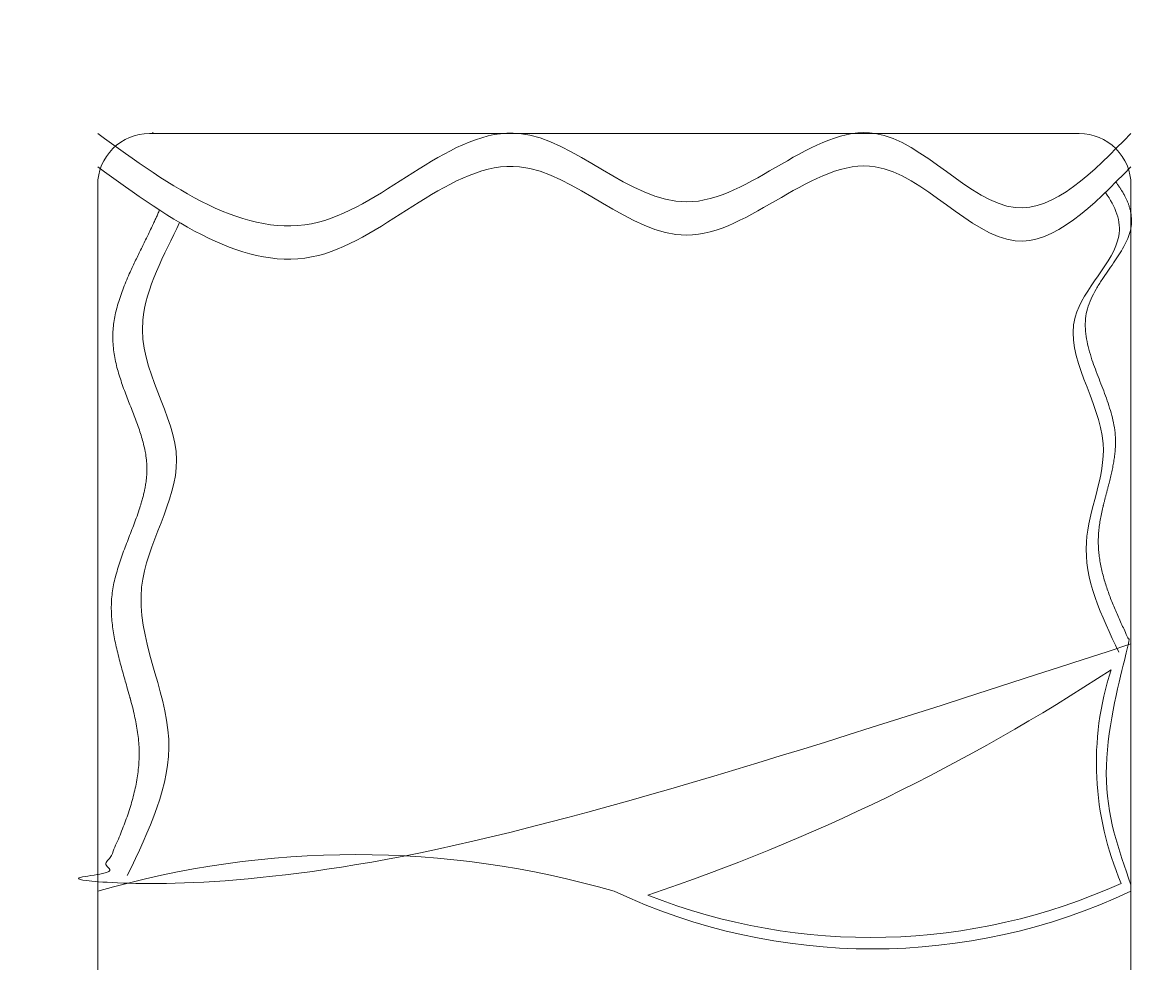
# Model space of a CAD drawing. Units: inches. Extents: x -61 to 1599, y -1316 to 257.
# Tile 188 of 204: x 1088 to 1163, y -391 to -328. Entities that reach past the tile are written whole.
import ezdxf

# ---------------------------------------------------------------- set-up
doc = ezdxf.new("R2010")
doc.units = ezdxf.units.IN
doc.header["$MEASUREMENT"] = 0
doc.layers.add('A-ANNO-DIMS', color=2, linetype='Continuous', lineweight=18)
doc.layers.add('FURNITURE', color=83, linetype='Continuous', lineweight=18)
doc.layers.add('LT', color=8, linetype='Continuous')
doc.styles.get("Standard").update_dxf_attribs({"font": 'arial.ttf'})
doc.dimstyles.get("Standard").update_dxf_attribs({"dimtxt": 0.18, "dimasz": 0.18, "dimexe": 0.18, "dimexo": 0.0625, "dimgap": 0.09, "dimtad": 0, "dimtih": 1, "dimtoh": 1, "dimdec": 0, "dimzin": 0, "dimdsep": 46, "dimlunit": 3, "dimtxsty": 'Standard', "dimcen": 0.09, "dimadec": 0, "dimazin": 0, "dimtfac": 1, "dimtdec": 0, "dimtofl": 0, "dimtmove": 0, "dimatfit": 3, "dimfxl": 1, "dimtolj": 1, "dimtzin": 0, "dimarcsym": 0})

# ---------------------------------------------------------------- blocks, each defined once
blk = doc.blocks.new('*U15')
at = {"layer": 'LT'}
blk.add_line((0, 0.175), (0, -0.175), dxfattribs=at)
for centre, start, end in [((0.509, 0), 160.9983, 199.0017), ((-0.509, 0), 340.9983, 19.0017)]:
    blk.add_arc(centre, 0.539, start, end, dxfattribs=at)
blk = doc.blocks.new('*U16')
at = {"layer": 'LT', "transparency": 16777216}
for p, rotation in [((-66.649, -18.828), 96), ((-66.642, -18.755), 72), ((-66.627, -18.897), 120), ((-66.605, -18.692), 48.00000000000001), ((-66.578, -18.951), 144), ((-66.546, -18.649), 24), ((-66.512, -18.981), 168.0000000000001), ((-66.439, -18.981), 192), ((-66.404, -18.649), 336.0000000000001), ((-66.372, -18.951), 216), ((-66.345, -18.692), 312), ((-66.323, -18.897), 240), ((-66.308, -18.755), 288.0000000000001), ((-66.301, -18.828), 264)]:
    blk.add_blockref('*U15', p, dxfattribs=dict(at, rotation=rotation))
blk.add_blockref('*U15', (-66.475, -18.634), dxfattribs=at)
blk = doc.blocks.new('*U45')
at = {"layer": 'LT'}
blk.add_line((0, 0.175), (0, -0.175), dxfattribs=at)
for centre, start, end in [((0.509, 0), 160.9983, 199.0017), ((-0.509, 0), 340.9983, 19.0017)]:
    blk.add_arc(centre, 0.539, start, end, dxfattribs=at)
blk = doc.blocks.new('*U46')
at = {"layer": 'LT', "transparency": 16777216}
for p, rotation in [((-66.649, -18.828), 96), ((-66.642, -18.755), 72), ((-66.627, -18.897), 120), ((-66.605, -18.692), 48.00000000000001), ((-66.578, -18.951), 144), ((-66.546, -18.649), 24), ((-66.512, -18.981), 168.0000000000001), ((-66.439, -18.981), 192), ((-66.404, -18.649), 336.0000000000001), ((-66.372, -18.951), 216), ((-66.345, -18.692), 312), ((-66.323, -18.897), 240), ((-66.308, -18.755), 288.0000000000001), ((-66.301, -18.828), 264)]:
    blk.add_blockref('*U45', p, dxfattribs=dict(at, rotation=rotation))
blk.add_blockref('*U45', (-66.475, -18.634), dxfattribs=at)
blk = doc.blocks.new('*U9')
at = {"layer": 'LT'}
blk.add_line((0, 0.175), (0, -0.175), dxfattribs=at)
for centre, start, end in [((0.509, 0), 160.9983, 199.0017), ((-0.509, 0), 340.9983, 19.0017)]:
    blk.add_arc(centre, 0.539, start, end, dxfattribs=at)
blk = doc.blocks.new('*U10')
at = {"layer": 'LT', "transparency": 16777216}
for p, rotation in [((-66.649, -18.828), 96), ((-66.642, -18.755), 72), ((-66.627, -18.897), 120), ((-66.605, -18.692), 48.00000000000001), ((-66.578, -18.951), 144), ((-66.546, -18.649), 24), ((-66.512, -18.981), 168.0000000000001), ((-66.439, -18.981), 192), ((-66.404, -18.649), 336.0000000000001), ((-66.372, -18.951), 216), ((-66.345, -18.692), 312), ((-66.323, -18.897), 240), ((-66.308, -18.755), 288.0000000000001), ((-66.301, -18.828), 264)]:
    blk.add_blockref('*U9', p, dxfattribs=dict(at, rotation=rotation))
blk.add_blockref('*U9', (-66.475, -18.634), dxfattribs=at)
blk = doc.blocks.new('*U39')
at = {"layer": 'LT'}
blk.add_line((0, 0.175), (0, -0.175), dxfattribs=at)
for centre, start, end in [((0.509, 0), 160.9983, 199.0017), ((-0.509, 0), 340.9983, 19.0017)]:
    blk.add_arc(centre, 0.539, start, end, dxfattribs=at)
blk = doc.blocks.new('*U40')
at = {"layer": 'LT', "transparency": 16777216}
for p, rotation in [((-66.649, -18.828), 96), ((-66.642, -18.755), 72), ((-66.627, -18.897), 120), ((-66.605, -18.692), 48.00000000000001), ((-66.578, -18.951), 144), ((-66.546, -18.649), 24), ((-66.512, -18.981), 168.0000000000001), ((-66.439, -18.981), 192), ((-66.404, -18.649), 336.0000000000001), ((-66.372, -18.951), 216), ((-66.345, -18.692), 312), ((-66.323, -18.897), 240), ((-66.308, -18.755), 288.0000000000001), ((-66.301, -18.828), 264)]:
    blk.add_blockref('*U39', p, dxfattribs=dict(at, rotation=rotation))
blk.add_blockref('*U39', (-66.475, -18.634), dxfattribs=at)
blk = doc.blocks.new('*U17')
at = {"layer": 'LT'}
blk.add_line((0, 0.412), (0, -0.412), dxfattribs=at)
for centre, start, end in [((1.198, 0), 160.9983, 199.0017), ((-1.198, 0), 340.9983, 19.0017)]:
    blk.add_arc(centre, 1.267, start, end, dxfattribs=at)
blk = doc.blocks.new('*U18')
at = {"layer": 'LT', "transparency": 16777216}
for p, rotation in [((-156.639, -43.959), 48.00000000000001), ((-156.501, -43.858), 24), ((-156.165, -43.858), 336.0000000000001), ((-156.027, -43.959), 312), ((-156.743, -44.278), 96), ((-156.725, -44.108), 72), ((-156.69, -44.441), 120), ((-156.575, -44.569), 144), ((-156.419, -44.639), 168), ((-156.247, -44.639), 192), ((-156.091, -44.569), 216), ((-155.976, -44.441), 240), ((-155.941, -44.108), 288.0000000000001), ((-155.923, -44.278), 264)]:
    blk.add_blockref('*U17', p, dxfattribs=dict(at, rotation=rotation))
blk.add_blockref('*U17', (-156.333, -43.823), dxfattribs=at)
blk = doc.blocks.new('*U33')
at = {"layer": 'LT'}
blk.add_line((0, 0.412), (0, -0.412), dxfattribs=at)
for centre, start, end in [((1.198, 0), 160.9983, 199.0017), ((-1.198, 0), 340.9983, 19.0017)]:
    blk.add_arc(centre, 1.267, start, end, dxfattribs=at)
blk = doc.blocks.new('*U34')
at = {"layer": 'LT', "transparency": 16777216}
for p, rotation in [((-156.639, -43.959), 48.00000000000001), ((-156.501, -43.858), 24), ((-156.165, -43.858), 336.0000000000001), ((-156.027, -43.959), 312), ((-156.743, -44.278), 96), ((-156.725, -44.108), 72), ((-156.69, -44.441), 120), ((-156.575, -44.569), 144), ((-156.419, -44.639), 168), ((-156.247, -44.639), 192), ((-156.091, -44.569), 216), ((-155.976, -44.441), 240), ((-155.941, -44.108), 288.0000000000001), ((-155.923, -44.278), 264)]:
    blk.add_blockref('*U33', p, dxfattribs=dict(at, rotation=rotation))
blk.add_blockref('*U33', (-156.333, -43.823), dxfattribs=at)
blk = doc.blocks.new('*U11')
at = {"layer": 'LT'}
blk.add_line((0, 0.739), (0, -0.739), dxfattribs=at)
for centre, start, end in [((2.147, 0), 160.9983, 199.0017), ((-2.147, 0), 340.9983, 19.0017)]:
    blk.add_arc(centre, 2.27, start, end, dxfattribs=at)
blk = doc.blocks.new('*U12')
at = {"layer": 'LT', "transparency": 16777216}
for p, rotation in [((-280.791, -78.801), 48.00000000000001), ((-280.542, -78.621), 23.99999999999999), ((-279.941, -78.621), 336.0000000000001), ((-279.692, -78.801), 312), ((-280.977, -79.373), 96), ((-280.945, -79.067), 72), ((-280.882, -79.665), 120), ((-280.676, -79.894), 144), ((-280.395, -80.019), 168), ((-280.088, -80.019), 191.9999999999999), ((-279.807, -79.894), 216), ((-279.602, -79.665), 240), ((-279.539, -79.067), 288.0000000000001), ((-279.507, -79.373), 264)]:
    blk.add_blockref('*U11', p, dxfattribs=dict(at, rotation=rotation))
blk.add_blockref('*U11', (-280.242, -78.557), dxfattribs=at)
blk = doc.blocks.new('*U28')
at = {"layer": 'LT'}
blk.add_line((0, 0.412), (0, -0.412), dxfattribs=at)
for centre, start, end in [((1.198, 0), 160.9983, 199.0017), ((-1.198, 0), 340.9983, 19.0017)]:
    blk.add_arc(centre, 1.267, start, end, dxfattribs=at)
blk = doc.blocks.new('*U44')
at = {"layer": 'LT', "transparency": 16777216}
for p, rotation in [((-156.639, -43.959), 48.00000000000001), ((-156.501, -43.858), 24), ((-156.165, -43.858), 336.0000000000001), ((-156.027, -43.959), 312), ((-156.743, -44.278), 96), ((-156.725, -44.108), 72), ((-156.69, -44.441), 120), ((-156.575, -44.569), 144), ((-156.419, -44.639), 168), ((-156.247, -44.639), 192), ((-156.091, -44.569), 216), ((-155.976, -44.441), 240), ((-155.941, -44.108), 288.0000000000001), ((-155.923, -44.278), 264)]:
    blk.add_blockref('*U28', p, dxfattribs=dict(at, rotation=rotation))
blk.add_blockref('*U28', (-156.333, -43.823), dxfattribs=at)
blk = doc.blocks.new('*U13')
at = {"layer": 'LT'}
blk.add_line((0, 0.412), (0, -0.412), dxfattribs=at)
for centre, start, end in [((1.198, 0), 160.9983, 199.0017), ((-1.198, 0), 340.9983, 19.0017)]:
    blk.add_arc(centre, 1.267, start, end, dxfattribs=at)
blk = doc.blocks.new('*U14')
at = {"layer": 'LT', "transparency": 16777216}
for p, rotation in [((-156.639, -43.959), 48.00000000000001), ((-156.501, -43.858), 24), ((-156.165, -43.858), 336.0000000000001), ((-156.027, -43.959), 312), ((-156.743, -44.278), 96), ((-156.725, -44.108), 72), ((-156.69, -44.441), 120), ((-156.575, -44.569), 144), ((-156.419, -44.639), 168), ((-156.247, -44.639), 192), ((-156.091, -44.569), 216), ((-155.976, -44.441), 240), ((-155.941, -44.108), 288.0000000000001), ((-155.923, -44.278), 264)]:
    blk.add_blockref('*U13', p, dxfattribs=dict(at, rotation=rotation))
blk.add_blockref('*U13', (-156.333, -43.823), dxfattribs=at)
blk = doc.blocks.new('*U19')
at = {"layer": 'LT'}
blk.add_line((0, 0.175), (0, -0.175), dxfattribs=at)
for centre, start, end in [((0.509, 0), 160.9983, 199.0017), ((-0.509, 0), 340.9983, 19.0017)]:
    blk.add_arc(centre, 0.539, start, end, dxfattribs=at)
blk = doc.blocks.new('*U6')
at = {"layer": 'LT', "transparency": 16777216}
for p, rotation in [((-66.649, -18.828), 96), ((-66.642, -18.755), 72), ((-66.627, -18.897), 120), ((-66.605, -18.692), 48.00000000000001), ((-66.578, -18.951), 144), ((-66.546, -18.649), 24), ((-66.512, -18.981), 168.0000000000001), ((-66.439, -18.981), 192), ((-66.404, -18.649), 336.0000000000001), ((-66.372, -18.951), 216), ((-66.345, -18.692), 312), ((-66.323, -18.897), 240), ((-66.308, -18.755), 288.0000000000001), ((-66.301, -18.828), 264)]:
    blk.add_blockref('*U19', p, dxfattribs=dict(at, rotation=rotation))
blk.add_blockref('*U19', (-66.475, -18.634), dxfattribs=at)
blk = doc.blocks.new('*U35')
at = {"layer": 'LT'}
blk.add_line((0, 0.175), (0, -0.175), dxfattribs=at)
for centre, start, end in [((0.509, 0), 160.9983, 199.0017), ((-0.509, 0), 340.9983, 19.0017)]:
    blk.add_arc(centre, 0.539, start, end, dxfattribs=at)
blk = doc.blocks.new('*U36')
at = {"layer": 'LT', "transparency": 16777216}
for p, rotation in [((-66.649, -18.828), 96), ((-66.642, -18.755), 72), ((-66.627, -18.897), 120), ((-66.605, -18.692), 48.00000000000001), ((-66.578, -18.951), 144), ((-66.546, -18.649), 24), ((-66.512, -18.981), 168.0000000000001), ((-66.439, -18.981), 192), ((-66.404, -18.649), 336.0000000000001), ((-66.372, -18.951), 216), ((-66.345, -18.692), 312), ((-66.323, -18.897), 240), ((-66.308, -18.755), 288.0000000000001), ((-66.301, -18.828), 264)]:
    blk.add_blockref('*U35', p, dxfattribs=dict(at, rotation=rotation))
blk.add_blockref('*U35', (-66.475, -18.634), dxfattribs=at)
blk = doc.blocks.new('*U7')
at = {"layer": 'LT'}
blk.add_line((0, 0.175), (0, -0.175), dxfattribs=at)
for centre, start, end in [((0.509, 0), 160.9983, 199.0017), ((-0.509, 0), 340.9983, 19.0017)]:
    blk.add_arc(centre, 0.539, start, end, dxfattribs=at)
blk = doc.blocks.new('*U8')
at = {"layer": 'LT', "transparency": 16777216}
for p, rotation in [((-66.649, -18.828), 96), ((-66.642, -18.755), 72), ((-66.627, -18.897), 120), ((-66.605, -18.692), 48.00000000000001), ((-66.578, -18.951), 144), ((-66.546, -18.649), 24), ((-66.512, -18.981), 168.0000000000001), ((-66.439, -18.981), 192), ((-66.404, -18.649), 336.0000000000001), ((-66.372, -18.951), 216), ((-66.345, -18.692), 312), ((-66.323, -18.897), 240), ((-66.308, -18.755), 288.0000000000001), ((-66.301, -18.828), 264)]:
    blk.add_blockref('*U7', p, dxfattribs=dict(at, rotation=rotation))
blk.add_blockref('*U7', (-66.475, -18.634), dxfattribs=at)
blk = doc.blocks.new('*U37')
at = {"layer": 'LT'}
blk.add_line((0, 0.175), (0, -0.175), dxfattribs=at)
for centre, start, end in [((0.509, 0), 160.9983, 199.0017), ((-0.509, 0), 340.9983, 19.0017)]:
    blk.add_arc(centre, 0.539, start, end, dxfattribs=at)
blk = doc.blocks.new('*U38')
at = {"layer": 'LT', "transparency": 16777216}
for p, rotation in [((-66.649, -18.828), 96), ((-66.642, -18.755), 72), ((-66.627, -18.897), 120), ((-66.605, -18.692), 48.00000000000001), ((-66.578, -18.951), 144), ((-66.546, -18.649), 24), ((-66.512, -18.981), 168.0000000000001), ((-66.439, -18.981), 192), ((-66.404, -18.649), 336.0000000000001), ((-66.372, -18.951), 216), ((-66.345, -18.692), 312), ((-66.323, -18.897), 240), ((-66.308, -18.755), 288.0000000000001), ((-66.301, -18.828), 264)]:
    blk.add_blockref('*U37', p, dxfattribs=dict(at, rotation=rotation))
blk.add_blockref('*U37', (-66.475, -18.634), dxfattribs=at)
blk = doc.blocks.new('*U3')
at = {"layer": 'LT'}
blk.add_line((0, 0.175), (0, -0.175), dxfattribs=at)
for centre, start, end in [((0.509, 0), 160.9983, 199.0017), ((-0.509, 0), 340.9983, 19.0017)]:
    blk.add_arc(centre, 0.539, start, end, dxfattribs=at)
blk = doc.blocks.new('*U4')
at = {"layer": 'LT', "transparency": 16777216}
for p, rotation in [((-66.649, -18.828), 96), ((-66.642, -18.755), 72), ((-66.627, -18.897), 120), ((-66.605, -18.692), 48.00000000000001), ((-66.578, -18.951), 144), ((-66.546, -18.649), 24), ((-66.512, -18.981), 168.0000000000001), ((-66.439, -18.981), 192), ((-66.404, -18.649), 336.0000000000001), ((-66.372, -18.951), 216), ((-66.345, -18.692), 312), ((-66.323, -18.897), 240), ((-66.308, -18.755), 288.0000000000001), ((-66.301, -18.828), 264)]:
    blk.add_blockref('*U3', p, dxfattribs=dict(at, rotation=rotation))
blk.add_blockref('*U3', (-66.475, -18.634), dxfattribs=at)
blk = doc.blocks.new('*U20')
at = {"layer": 'LT'}
blk.add_line((0, 0.175), (0, -0.175), dxfattribs=at)
for centre, start, end in [((0.509, 0), 160.9983, 199.0017), ((-0.509, 0), 340.9983, 19.0017)]:
    blk.add_arc(centre, 0.539, start, end, dxfattribs=at)
blk = doc.blocks.new('*U21')
at = {"layer": 'LT', "transparency": 16777216}
for p, rotation in [((-66.649, -18.828), 96), ((-66.642, -18.755), 72), ((-66.627, -18.897), 120), ((-66.605, -18.692), 48.00000000000001), ((-66.578, -18.951), 144), ((-66.546, -18.649), 24), ((-66.512, -18.981), 168.0000000000001), ((-66.439, -18.981), 192), ((-66.404, -18.649), 336.0000000000001), ((-66.372, -18.951), 216), ((-66.345, -18.692), 312), ((-66.323, -18.897), 240), ((-66.308, -18.755), 288.0000000000001), ((-66.301, -18.828), 264)]:
    blk.add_blockref('*U20', p, dxfattribs=dict(at, rotation=rotation))
blk.add_blockref('*U20', (-66.475, -18.634), dxfattribs=at)
blk = doc.blocks.new('*U52')
at = {"layer": 'LT'}
blk.add_line((0, 0.175), (0, -0.175), dxfattribs=at)
for centre, start, end in [((0.509, 0), 160.9983, 199.0017), ((-0.509, 0), 340.9983, 19.0017)]:
    blk.add_arc(centre, 0.539, start, end, dxfattribs=at)
blk = doc.blocks.new('*U53')
at = {"layer": 'LT', "transparency": 16777216}
for p, rotation in [((-66.649, -18.828), 96), ((-66.642, -18.755), 72), ((-66.627, -18.897), 120), ((-66.605, -18.692), 48.00000000000001), ((-66.578, -18.951), 144), ((-66.546, -18.649), 24), ((-66.512, -18.981), 168.0000000000001), ((-66.439, -18.981), 192), ((-66.404, -18.649), 336.0000000000001), ((-66.372, -18.951), 216), ((-66.345, -18.692), 312), ((-66.323, -18.897), 240), ((-66.308, -18.755), 288.0000000000001), ((-66.301, -18.828), 264)]:
    blk.add_blockref('*U52', p, dxfattribs=dict(at, rotation=rotation))
blk.add_blockref('*U52', (-66.475, -18.634), dxfattribs=at)
blk = doc.blocks.new('*U29')
at = {"layer": 'LT'}
blk.add_line((0, 0.175), (0, -0.175), dxfattribs=at)
for centre, start, end in [((0.509, 0), 160.9983, 199.0017), ((-0.509, 0), 340.9983, 19.0017)]:
    blk.add_arc(centre, 0.539, start, end, dxfattribs=at)
blk = doc.blocks.new('*U30')
at = {"layer": 'LT', "transparency": 16777216}
for p, rotation in [((-66.649, -18.828), 96), ((-66.642, -18.755), 72), ((-66.627, -18.897), 120), ((-66.605, -18.692), 48.00000000000001), ((-66.578, -18.951), 144), ((-66.546, -18.649), 24), ((-66.512, -18.981), 168.0000000000001), ((-66.439, -18.981), 192), ((-66.404, -18.649), 336.0000000000001), ((-66.372, -18.951), 216), ((-66.345, -18.692), 312), ((-66.323, -18.897), 240), ((-66.308, -18.755), 288.0000000000001), ((-66.301, -18.828), 264)]:
    blk.add_blockref('*U29', p, dxfattribs=dict(at, rotation=rotation))
blk.add_blockref('*U29', (-66.475, -18.634), dxfattribs=at)
blk = doc.blocks.new('*U5')
at = {"layer": 'LT'}
blk.add_line((0, 0.412), (0, -0.412), dxfattribs=at)
for centre, start, end in [((1.198, 0), 160.9983, 199.0017), ((-1.198, 0), 340.9983, 19.0017)]:
    blk.add_arc(centre, 1.267, start, end, dxfattribs=at)
blk = doc.blocks.new('*U47')
at = {"layer": 'LT', "transparency": 16777216}
for p, rotation in [((-156.639, -43.959), 48.00000000000001), ((-156.501, -43.858), 24), ((-156.165, -43.858), 336.0000000000001), ((-156.027, -43.959), 312), ((-156.743, -44.278), 96), ((-156.725, -44.108), 72), ((-156.69, -44.441), 120), ((-156.575, -44.569), 144), ((-156.419, -44.639), 168), ((-156.247, -44.639), 192), ((-156.091, -44.569), 216), ((-155.976, -44.441), 240), ((-155.941, -44.108), 288.0000000000001), ((-155.923, -44.278), 264)]:
    blk.add_blockref('*U5', p, dxfattribs=dict(at, rotation=rotation))
blk.add_blockref('*U5', (-156.333, -43.823), dxfattribs=at)
blk = doc.blocks.new('*U22')
at = {"layer": 'LT'}
blk.add_line((0, 0.412), (0, -0.412), dxfattribs=at)
for centre, start, end in [((1.198, 0), 160.9983, 199.0017), ((-1.198, 0), 340.9983, 19.0017)]:
    blk.add_arc(centre, 1.267, start, end, dxfattribs=at)
blk = doc.blocks.new('*U23')
at = {"layer": 'LT', "transparency": 16777216}
for p, rotation in [((-156.639, -43.959), 48.00000000000001), ((-156.501, -43.858), 24), ((-156.165, -43.858), 336.0000000000001), ((-156.027, -43.959), 312), ((-156.743, -44.278), 96), ((-156.725, -44.108), 72), ((-156.69, -44.441), 120), ((-156.575, -44.569), 144), ((-156.419, -44.639), 168), ((-156.247, -44.639), 192), ((-156.091, -44.569), 216), ((-155.976, -44.441), 240), ((-155.941, -44.108), 288.0000000000001), ((-155.923, -44.278), 264)]:
    blk.add_blockref('*U22', p, dxfattribs=dict(at, rotation=rotation))
blk.add_blockref('*U22', (-156.333, -43.823), dxfattribs=at)
blk = doc.blocks.new('*U54')
at = {"layer": 'LT'}
blk.add_line((0, 0.739), (0, -0.739), dxfattribs=at)
for centre, start, end in [((2.147, 0), 160.9983, 199.0017), ((-2.147, 0), 340.9983, 19.0017)]:
    blk.add_arc(centre, 2.27, start, end, dxfattribs=at)
blk = doc.blocks.new('*U41')
at = {"layer": 'LT', "transparency": 16777216}
for p, rotation in [((-280.791, -78.801), 48.00000000000001), ((-280.542, -78.621), 23.99999999999999), ((-279.941, -78.621), 336.0000000000001), ((-279.692, -78.801), 312), ((-280.977, -79.373), 96), ((-280.945, -79.067), 72), ((-280.882, -79.665), 120), ((-280.676, -79.894), 144), ((-280.395, -80.019), 168), ((-280.088, -80.019), 191.9999999999999), ((-279.807, -79.894), 216), ((-279.602, -79.665), 240), ((-279.539, -79.067), 288.0000000000001), ((-279.507, -79.373), 264)]:
    blk.add_blockref('*U54', p, dxfattribs=dict(at, rotation=rotation))
blk.add_blockref('*U54', (-280.242, -78.557), dxfattribs=at)
blk = doc.blocks.new('*U42')
at = {"layer": 'LT'}
blk.add_line((0, 0.412), (0, -0.412), dxfattribs=at)
for centre, start, end in [((1.198, 0), 160.9983, 199.0017), ((-1.198, 0), 340.9983, 19.0017)]:
    blk.add_arc(centre, 1.267, start, end, dxfattribs=at)
blk = doc.blocks.new('*U43')
at = {"layer": 'LT', "transparency": 16777216}
for p, rotation in [((-156.639, -43.959), 48.00000000000001), ((-156.501, -43.858), 24), ((-156.165, -43.858), 336.0000000000001), ((-156.027, -43.959), 312), ((-156.743, -44.278), 96), ((-156.725, -44.108), 72), ((-156.69, -44.441), 120), ((-156.575, -44.569), 144), ((-156.419, -44.639), 168), ((-156.247, -44.639), 192), ((-156.091, -44.569), 216), ((-155.976, -44.441), 240), ((-155.941, -44.108), 288.0000000000001), ((-155.923, -44.278), 264)]:
    blk.add_blockref('*U42', p, dxfattribs=dict(at, rotation=rotation))
blk.add_blockref('*U42', (-156.333, -43.823), dxfattribs=at)
blk = doc.blocks.new('*U31')
at = {"layer": 'LT'}
blk.add_line((0, 0.412), (0, -0.412), dxfattribs=at)
for centre, start, end in [((1.198, 0), 160.9983, 199.0017), ((-1.198, 0), 340.9983, 19.0017)]:
    blk.add_arc(centre, 1.267, start, end, dxfattribs=at)
blk = doc.blocks.new('*U32')
at = {"layer": 'LT', "transparency": 16777216}
for p, rotation in [((-156.639, -43.959), 48.00000000000001), ((-156.501, -43.858), 24), ((-156.165, -43.858), 336.0000000000001), ((-156.027, -43.959), 312), ((-156.743, -44.278), 96), ((-156.725, -44.108), 72), ((-156.69, -44.441), 120), ((-156.575, -44.569), 144), ((-156.419, -44.639), 168), ((-156.247, -44.639), 192), ((-156.091, -44.569), 216), ((-155.976, -44.441), 240), ((-155.941, -44.108), 288.0000000000001), ((-155.923, -44.278), 264)]:
    blk.add_blockref('*U31', p, dxfattribs=dict(at, rotation=rotation))
blk.add_blockref('*U31', (-156.333, -43.823), dxfattribs=at)
blk = doc.blocks.new('*U48')
at = {"layer": 'LT'}
blk.add_line((0, 0.175), (0, -0.175), dxfattribs=at)
for centre, start, end in [((0.509, 0), 160.9983, 199.0017), ((-0.509, 0), 340.9983, 19.0017)]:
    blk.add_arc(centre, 0.539, start, end, dxfattribs=at)
blk = doc.blocks.new('*U49')
at = {"layer": 'LT', "transparency": 16777216}
for p, rotation in [((-66.649, -18.828), 96), ((-66.642, -18.755), 72), ((-66.627, -18.897), 120), ((-66.605, -18.692), 48.00000000000001), ((-66.578, -18.951), 144), ((-66.546, -18.649), 24), ((-66.512, -18.981), 168.0000000000001), ((-66.439, -18.981), 192), ((-66.404, -18.649), 336.0000000000001), ((-66.372, -18.951), 216), ((-66.345, -18.692), 312), ((-66.323, -18.897), 240), ((-66.308, -18.755), 288.0000000000001), ((-66.301, -18.828), 264)]:
    blk.add_blockref('*U48', p, dxfattribs=dict(at, rotation=rotation))
blk.add_blockref('*U48', (-66.475, -18.634), dxfattribs=at)
blk = doc.blocks.new('*U24')
at = {"layer": 'LT'}
blk.add_line((0, 0.175), (0, -0.175), dxfattribs=at)
for centre, start, end in [((0.509, 0), 160.9983, 199.0017), ((-0.509, 0), 340.9983, 19.0017)]:
    blk.add_arc(centre, 0.539, start, end, dxfattribs=at)
blk = doc.blocks.new('*U25')
at = {"layer": 'LT', "transparency": 16777216}
for p, rotation in [((-66.649, -18.828), 96), ((-66.642, -18.755), 72), ((-66.627, -18.897), 120), ((-66.605, -18.692), 48.00000000000001), ((-66.578, -18.951), 144), ((-66.546, -18.649), 24), ((-66.512, -18.981), 168.0000000000001), ((-66.439, -18.981), 192), ((-66.404, -18.649), 336.0000000000001), ((-66.372, -18.951), 216), ((-66.345, -18.692), 312), ((-66.323, -18.897), 240), ((-66.308, -18.755), 288.0000000000001), ((-66.301, -18.828), 264)]:
    blk.add_blockref('*U24', p, dxfattribs=dict(at, rotation=rotation))
blk.add_blockref('*U24', (-66.475, -18.634), dxfattribs=at)
blk = doc.blocks.new('*U50')
at = {"layer": 'LT'}
blk.add_line((0, 0.175), (0, -0.175), dxfattribs=at)
for centre, start, end in [((0.509, 0), 160.9983, 199.0017), ((-0.509, 0), 340.9983, 19.0017)]:
    blk.add_arc(centre, 0.539, start, end, dxfattribs=at)
blk = doc.blocks.new('*U51')
at = {"layer": 'LT', "transparency": 16777216}
for p, rotation in [((-66.649, -18.828), 96), ((-66.642, -18.755), 72), ((-66.627, -18.897), 120), ((-66.605, -18.692), 48.00000000000001), ((-66.578, -18.951), 144), ((-66.546, -18.649), 24), ((-66.512, -18.981), 168.0000000000001), ((-66.439, -18.981), 192), ((-66.404, -18.649), 336.0000000000001), ((-66.372, -18.951), 216), ((-66.345, -18.692), 312), ((-66.323, -18.897), 240), ((-66.308, -18.755), 288.0000000000001), ((-66.301, -18.828), 264)]:
    blk.add_blockref('*U50', p, dxfattribs=dict(at, rotation=rotation))
blk.add_blockref('*U50', (-66.475, -18.634), dxfattribs=at)
blk = doc.blocks.new('*U26')
at = {"layer": 'LT'}
blk.add_line((0, 0.175), (0, -0.175), dxfattribs=at)
for centre, start, end in [((0.509, 0), 160.9983, 199.0017), ((-0.509, 0), 340.9983, 19.0017)]:
    blk.add_arc(centre, 0.539, start, end, dxfattribs=at)
blk = doc.blocks.new('*U27')
at = {"layer": 'LT', "transparency": 16777216}
for p, rotation in [((-66.649, -18.828), 96), ((-66.642, -18.755), 72), ((-66.627, -18.897), 120), ((-66.605, -18.692), 48.00000000000001), ((-66.578, -18.951), 144), ((-66.546, -18.649), 24), ((-66.512, -18.981), 168.0000000000001), ((-66.439, -18.981), 192), ((-66.404, -18.649), 336.0000000000001), ((-66.372, -18.951), 216), ((-66.345, -18.692), 312), ((-66.323, -18.897), 240), ((-66.308, -18.755), 288.0000000000001), ((-66.301, -18.828), 264)]:
    blk.add_blockref('*U26', p, dxfattribs=dict(at, rotation=rotation))
blk.add_blockref('*U26', (-66.475, -18.634), dxfattribs=at)
blk = doc.blocks.new('BED-DOUBLE')
for p, q in [((1.272, 20.467), (70.263, 20.467)), ((1.272, 19.317), (70.263, 19.317)), ((10.471, 1.379), (10.471, 16.557)), ((34.388, 16.557), (10.471, 16.557)), ((10.471, 16.557), (13.35, 15.18)), ((10.471, 16.557), (14.039, 13.107)), ((10.471, 16.557), (12.454, 13.305)), ((34.388, 16.557), (30.82, 13.107)), ((34.388, 16.557), (31.508, 15.18)), ((34.388, 16.557), (32.405, 13.305)), ((37.147, 1.379), (37.147, 16.557)), ((61.064, 16.557), (37.147, 16.557)), ((37.147, 16.557), (40.027, 15.18)), ((37.147, 16.557), (40.715, 13.107)), ((37.147, 16.557), (39.13, 13.305)), ((61.064, 16.557), (57.496, 13.107)), ((61.064, 16.557), (58.185, 15.18)), ((61.064, 16.557), (59.081, 13.305)), ((13.35, 15.18), (13.35, 14.829)), ((31.508, 15.18), (31.508, 14.829)), ((40.027, 15.18), (40.027, 14.829)), ((58.185, 15.18), (58.185, 14.829)), ((12.454, 13.305), (12.454, 12.955)), ((14.052, 13.149), (14.052, 12.324)), ((30.806, 13.149), (30.806, 12.324)), ((32.405, 13.305), (32.405, 12.955)), ((39.13, 13.305), (39.13, 12.955)), ((40.729, 13.149), (40.729, 12.324)), ((57.483, 13.149), (57.483, 12.324)), ((59.081, 13.305), (59.081, 12.955)), ((22.429, 8.968), (22.429, 10.447)), ((49.106, 8.968), (49.106, 10.447)), ((14.052, 4.788), (14.052, 5.613)), ((30.806, 4.788), (30.806, 5.613)), ((40.729, 4.788), (40.729, 5.613)), ((57.483, 4.788), (57.483, 5.613)), ((10.471, 1.379), (14.039, 4.83)), ((10.471, 1.379), (12.454, 4.631)), ((12.454, 4.631), (12.454, 4.982)), ((34.388, 1.379), (30.82, 4.83)), ((32.405, 4.631), (32.405, 4.982)), ((34.388, 1.379), (32.405, 4.631)), ((37.147, 1.379), (40.715, 4.83)), ((37.147, 1.379), (39.13, 4.631)), ((39.13, 4.631), (39.13, 4.982)), ((61.064, 1.379), (57.496, 4.83)), ((59.081, 4.631), (59.081, 4.982)), ((61.064, 1.379), (59.081, 4.631)), ((13.35, 2.756), (13.35, 3.107)), ((31.508, 2.756), (31.508, 3.107)), ((40.027, 2.756), (40.027, 3.107)), ((58.185, 2.756), (58.185, 3.107)), ((10.471, 1.379), (13.35, 2.756)), ((34.388, 1.379), (31.508, 2.756)), ((37.147, 1.379), (40.027, 2.756)), ((61.064, 1.379), (58.185, 2.756)), ((34.388, 1.379), (34.388, 1.379)), ((61.064, 1.379), (61.064, 1.379))]:
    blk.add_line(p, q)
for points in [[(1.272, 88.537), (1.272, 3.449, 0.414214), (4.722, 0), (66.813, 0, 0.414214), (70.263, 3.449), (70.263, 88.537, 0.414214), (66.813, 91.987), (4.722, 91.987, 0.414214)], [(38.01, 41.126, 0.064396), (68.933, 56.181, 0.181766), (69.614, 41.916, -0.202767)], [(13.35, 15.18, 0.167358), (13.35, 14.829, 0.167358)], [(40.027, 15.18, 0.167358), (40.027, 14.829, 0.167358)], [(12.454, 13.305, 0.167358), (12.454, 12.955, 0.167358)], [(14.052, 13.149, 0.167358), (14.052, 12.324, 0.167358)], [(30.806, 12.324, 0.167358), (30.806, 13.149, 0.167358)], [(32.405, 12.955, 0.167358), (32.405, 13.305, 0.167358)], [(39.13, 13.305, 0.167358), (39.13, 12.955, 0.167358)], [(40.729, 13.149, 0.167358), (40.729, 12.324, 0.167358)], [(57.483, 12.324, 0.167358), (57.483, 13.149, 0.167358)], [(59.081, 12.955, 0.167358), (59.081, 13.305, 0.167358)], [(22.429, 8.968, 0.167358), (22.429, 10.447, 0.167358)], [(49.106, 8.968, 0.167358), (49.106, 10.447, 0.167358)], [(14.052, 5.613, 0.167358), (14.052, 4.788, 0.167358)], [(30.806, 4.788, 0.167358), (30.806, 5.613, 0.167358)], [(40.729, 5.613, 0.167358), (40.729, 4.788, 0.167358)], [(57.483, 4.788, 0.167358), (57.483, 5.613, 0.167358)], [(12.454, 4.982, 0.167358), (12.454, 4.631, 0.167358)], [(32.405, 4.631, 0.167358), (32.405, 4.982, 0.167358)], [(39.13, 4.982, 0.167358), (39.13, 4.631, 0.167358)], [(59.081, 4.631, 0.167358), (59.081, 4.982, 0.167358)], [(13.35, 3.107, 0.167358), (13.35, 2.756, 0.167358)], [(31.508, 2.756, 0.167358), (31.508, 3.107, 0.167358)], [(40.027, 3.107, 0.167358), (40.027, 2.756, 0.167358)], [(58.185, 2.756, 0.167358), (58.185, 3.107, 0.167358)]]:
    blk.add_lwpolyline(points, format="xyb", close=True)
blk.add_lwpolyline([(70.263, 41.387, -0.22309), (35.767, 41.387, 0.142156), (1.272, 41.387)], format="xyb")
for points in [[(34.388, 16.557), (34.388, 1.379), (10.471, 1.379), (10.471, 16.557), (34.388, 16.557), (34.388, 1.379), (10.471, 1.379)], [(61.064, 16.557), (61.064, 1.379), (37.147, 1.379)]]:
    blk.add_lwpolyline(points)
for centre, radius in [((13.35, 15.18), 0.351), ((31.508, 15.18), 0.351), ((40.027, 15.18), 0.351), ((58.185, 15.18), 0.351), ((12.454, 13.305), 0.351), ((14.052, 13.149), 0.825), ((30.806, 13.149), 0.825), ((32.405, 13.305), 0.351), ((39.13, 13.305), 0.351), ((40.729, 13.149), 0.825), ((57.483, 13.149), 0.825), ((59.081, 13.305), 0.351), ((22.429, 8.968), 1.982), ((49.106, 8.968), 1.982), ((22.429, 8.968), 1.478), ((49.106, 8.968), 1.478), ((14.052, 4.788), 0.825), ((30.806, 4.788), 0.825), ((40.729, 4.788), 0.825), ((57.483, 4.788), 0.825), ((12.454, 4.631), 0.351), ((32.405, 4.631), 0.351), ((39.13, 4.631), 0.351), ((59.081, 4.631), 0.351), ((13.35, 2.756), 0.351), ((31.508, 2.756), 0.351), ((40.027, 2.756), 0.351), ((58.185, 2.756), 0.351)]:
    blk.add_circle(centre, radius)
for centre, radius, start, end in [((-16.003, 8.968), 27.54, 344.0046, 15.9954), ((22.429, 74.54), 59.203, 258.34678, 281.65322), ((60.861, 8.968), 27.54, 164.0046, 195.9954), ((10.674, 8.968), 27.54, 344.0046, 15.9954), ((49.106, 74.54), 59.203, 258.34678, 281.65322), ((87.538, 8.968), 27.54, 164.0046, 195.9954), ((32.017, 15.005), 0.539, 160.9983, 199.0017), ((30.999, 15.005), 0.539, 340.9983, 19.0017), ((58.694, 15.005), 0.539, 160.9983, 199.0017), ((57.675, 15.005), 0.539, 340.9983, 19.0017), ((22.429, -56.603), 59.203, 78.34678, 101.65322), ((49.106, -56.603), 59.203, 78.34678, 101.65322)]:
    blk.add_arc(centre, radius, start, end)
for points, knots in [([(70.263, 91.987), (67.707, 89.379), (62.206, 83.764), (52.487, 96.724), (40.92, 82.741), (28.609, 96.737), (15.695, 81.527), (6.205, 88.409), (1.272, 91.987)], [0, 0, 0, 0, 9.176033, 19.753992, 33.150145, 45.209422, 59.881559, 75.764594, 75.764594, 75.764594, 75.764594]), ([(70.263, 89.765), (67.707, 87.157), (62.206, 81.542), (52.487, 94.502), (40.92, 80.519), (28.609, 94.515), (15.695, 79.305), (6.205, 86.187), (1.272, 89.765)], [0, 0, 0, 0, 9.176033, 19.753992, 33.150145, 45.209422, 59.881559, 75.764594, 75.764594, 75.764594, 75.764594]), ([(69.451, 57.362), (68.289, 59.79), (66.113, 64.336), (70.043, 71.905), (64.118, 79.112), (70.314, 84.4), (69.244, 87.088), (68.552, 88.052)], [0, 0, 0, 0, 6.649676, 12.451782, 19.973966, 25.324174, 28.349676, 28.349676, 28.349676, 28.349676]), ([(3.252, 42.437), (4.702, 45.448), (7.724, 51.72), (2.116, 61.25), (8.808, 70.52), (2.434, 77.934), (5.722, 83.908), (6.746, 86.037)], [0, 0, 0, 0, 8.27671, 17.241866, 24.903358, 33.244933, 38.427294, 38.427294, 38.427294, 38.427294])]:
    blk.add_open_spline(points, degree=3, knots=knots)
blk.add_open_spline([(5.011, 91.987), (4.986, 92.006), (4.961, 92.025), (4.936, 92.044)], degree=3)
for points, weights, knots in [([(70.263, 41.825), (68.018, 47.029), (68.018, 52.696), (70.263, 57.9), (69.1, 60.328), (66.924, 64.874), (70.854, 72.444), (64.929, 79.65), (71.186, 84.991), (70.014, 87.727), (69.253, 88.741)], [1, 0.945466318698, 0.945466318698, 1, 1, 1, 1, 1, 1, 1, 1], [0, 0, 0, 0, 0.814571, 0.814571, 0.814571, 7.464247, 13.266353, 20.788537, 26.138745, 29.321895, 29.321895, 29.321895, 29.321895]), ([(70.263, 57.9), (59.862, 50.943), (48.595, 45.5), (36.681, 41.677), (36.463, 41.771), (36.247, 41.868), (36.032, 41.966), (24.597, 45.284), (12.692, 45.258), (1.272, 41.889), (2.723, 44.9), (5.745, 51.172), (0.137, 60.702), (6.828, 69.972), (0.109, 77.787), (4.354, 84.383), (5.398, 86.876)], [1, 0.993520320424, 0.993520320424, 1, 0.99997444972, 0.99997444972, 1, 0.973174868659, 0.973174868659, 1, 1, 1, 1, 1, 1, 1, 1], [0, 0, 0, 0, 0.279074, 0.279074, 0.279074, 0.296584, 0.296584, 0.296584, 0.865868, 0.865868, 0.865868, 9.142578, 18.107734, 25.769226, 34.110801, 40.441511, 40.441511, 40.441511, 40.441511])]:
    blk.add_rational_spline(points, weights, degree=3, knots=knots)
for name, p in [('*U40', (79.825, 33.99)), ('*U30', (106.502, 33.99)), ('*U46', (78.929, 32.115)), ('*U34', (170.385, 57.384)), ('*U21', (105.605, 32.115)), ('*U23', (197.062, 57.384))]:
    blk.add_blockref(name, p)
at = {"extrusion": (0, 0, -1), "zscale": -1}
for name, p in [('*U36', (34.967, 33.99)), ('*U25', (8.291, 33.99)), ('*U14', (125.527, 57.384)), ('*U38', (34.07, 32.115)), ('*U32', (98.85, 57.384)), ('*U27', (7.394, 32.115))]:
    blk.add_blockref(name, p, dxfattribs=at)
at = {"rotation": 180}
for name, p in [('*U12', (-257.812, -70.328)), ('*U41', (-231.136, -70.328)), ('*U44', (-125.527, -39.447)), ('*U43', (-98.85, -39.447)), ('*U8', (-34.07, -14.178)), ('*U51', (-7.394, -14.178)), ('*U6', (-34.967, -16.053)), ('*U49', (-8.291, -16.053))]:
    blk.add_blockref(name, p, dxfattribs=at)
at = {"extrusion": (0, 0, -1), "zscale": -1, "rotation": 180}
for name, p in [('*U18', (-170.385, -39.447)), ('*U47', (-197.062, -39.447)), ('*U16', (-78.929, -14.178)), ('*U4', (-105.605, -14.178)), ('*U10', (-79.825, -16.053)), ('*U53', (-106.502, -16.053))]:
    blk.add_blockref(name, p, dxfattribs=at)
blk = doc.blocks.new('*D698')
at = {"layer": 'A-ANNO-DIMS', "color": 0, "lineweight": -2, "transparency": 16777216}
for p, q in [((644.765, -167.169), (1598.483, -167.169)), ((1598.303, -167.349), (1598.303, -363.987)), ((1598.303, -560.989), (1598.303, -364.351)), ((644.765, -561.169), (1598.483, -561.169))]:
    blk.add_line(p, q, dxfattribs=at)
at = {"layer": 'A-ANNO-DIMS', "color": 0, "transparency": 16777216}
for points in [[(1598.273, -167.349), (1598.333, -167.349), (1598.303, -167.169)], [(1598.273, -560.989), (1598.333, -560.989), (1598.303, -561.169)]]:
    blk.add_solid(points, dxfattribs=at)
at = {"layer": 'DEFPOINTS', "color": 0, "transparency": 16777216}
for p in [(644.703, -167.169), (1598.303, -167.169), (644.703, -561.169)]:
    blk.add_point(p, dxfattribs=at)
at = {"layer": 'A-ANNO-DIMS', "color": 0, "transparency": 16777216, "insert": (1598.303, -364.169), "char_height": 0.18, "attachment_point": 5}
blk.add_mtext('\\A1;394', dxfattribs=at)

msp = doc.modelspace()

# ---------------------------------------------------------------- block references
at = {"layer": 'FURNITURE'}
msp.add_blockref('BED-DOUBLE', (1091.2612, -427.6961), dxfattribs=at)

# ---------------------------------------------------------------- dimensions: what is measured, and where the dimension line sits
at = {"layer": 'A-ANNO-DIMS'}
dim = msp.add_linear_dim(base=(1598.3028, -167.169), p1=(644.7028, -561.169), p2=(644.7028, -167.169), angle=90, dimstyle='Standard', override={"dimdec": 0, "dimlfac": 1, "dimrnd": 0, "dimzin": 0, "dimdsep": 46, "dimlunit": 2}, dxfattribs=at)
dim.commit()
dim.dimension.update_dxf_attribs({"geometry": '*D698', "text_midpoint": (1598.3028, -364.169)})

doc.saveas('drawing.dxf')
